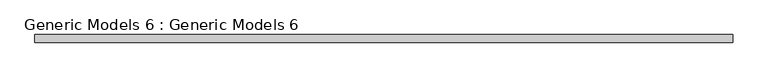
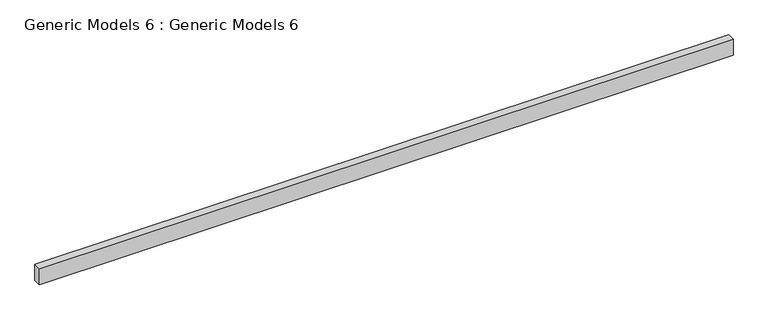
"""IFC4 building model written with IfcOpenShell, lengths in millimetres: proxy geometry, Generic Models 6 : Generic Models 6."""

from ifc_helpers import new_model, si_unit, frame, origin, place, context, project, spatial, polyline, outline, extrude, source, transform, mapped, element, save


def generic_models_6_generic_models_6_95f07958(model_context):
    return source(origin(), model_context, "Body", "SweptSolid", [
        extrude(outline(polyline([(12604.4370151, -3746.0004242), (12604.4370151, -3980.2775898), (-8934.7629849, -3980.2775898), (-8934.7629849, -3746.0004242), (12604.4370151, -3746.0004242)])), frame((0.0, 0.0, 12773.5804985), z_axis=(0.0, 0.0, 1.0), x_axis=(1.0, 0.0, 0.0)), (0.0, 0.0, 1.0), 532.0007846),
    ])


if __name__ == "__main__":
    model = new_model("IFC4")
    model_context = context("Model", 3, world=origin())
    ifc_project = project(units=[si_unit("LENGTHUNIT", "METRE", prefix="MILLI")], contexts=[model_context])
    site = spatial("IfcSite", under=ifc_project)
    building = spatial("IfcBuilding", under=site)
    placement = place(None, origin())
    generic_models_6_generic_models_6_shape = generic_models_6_generic_models_6_95f07958(model_context)
    element("IfcBuildingElementProxy", 1, Name="Generic Models 6 : Generic Models 6", ObjectType="Generic Models 6 : Generic Models 6", at=placement, inside=building, context=model_context, shape_type="MappedRepresentation", body=[
        mapped(generic_models_6_generic_models_6_shape, transform((0.0, 0.0, 0.0), x_axis=(1.0, 0.0, 0.0), y_axis=(0.0, 1.0, 0.0), z_axis=(0.0, 0.0, 1.0))),
    ])
    save(model, "model.ifc")
